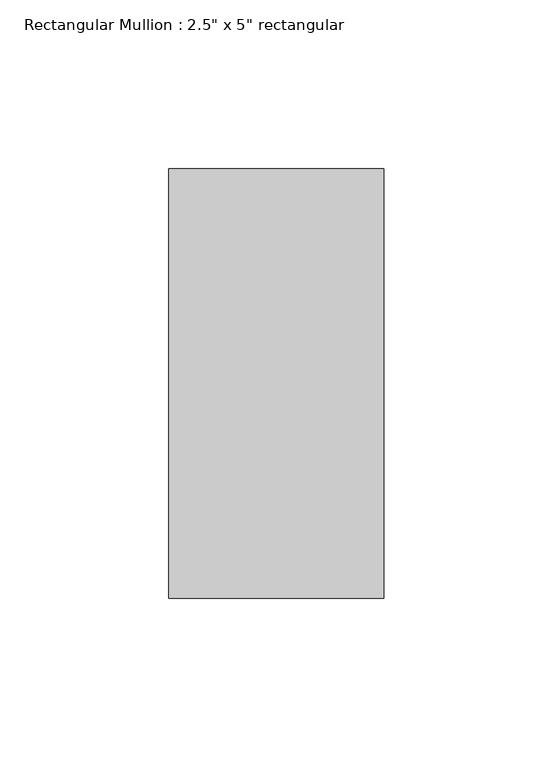
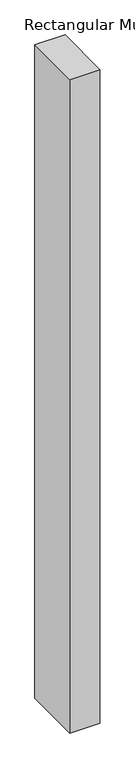
"""IFC4 building model written with IfcOpenShell, lengths in millimetres: member geometry."""

from ifc_helpers import new_model, si_unit, frame, origin, place, context, project, spatial, polyline, outline, extrude, source, transform, mapped, element, save


def member_b9522cbe(model_context):
    return source(origin(), model_context, "Body", "SweptSolid", [
        extrude(outline(polyline([(0.0, 63.5), (0.0, -63.5), (-63.5, -63.5), (-63.5, 63.5), (0.0, 63.5)])), frame((0.0, 0.0, -1452.5193485), z_axis=(0.0, 0.0, 1.0), x_axis=(1.0, 0.0, 0.0)), (0.0, 0.0, 1.0), 1452.5193485),
    ])


if __name__ == "__main__":
    model = new_model("IFC4")
    model_context = context("Model", 3, world=origin())
    ifc_project = project(units=[si_unit("LENGTHUNIT", "METRE", prefix="MILLI")], contexts=[model_context])
    site = spatial("IfcSite", under=ifc_project)
    building = spatial("IfcBuilding", under=site)
    placement = place(None, origin())
    member_shape = member_b9522cbe(model_context)
    element("IfcMember", 1, ObjectType="Rectangular Mullion : 2.5\" x 5\" rectangular", at=placement, inside=building, context=model_context, shape_type="MappedRepresentation", body=[
        mapped(member_shape, transform((0.0, 0.0, 0.0), x_axis=(1.0, 0.0, 0.0), y_axis=(0.0, 1.0, 0.0), z_axis=(0.0, 0.0, 1.0))),
    ])
    save(model, "model.ifc")

# Revit data of these elements
# Type "Rectangular Mullion : 2.5\" x 5\" rectangular"
#   built-in parameter 1007304 = 0.416667 (stored number, unit not read)
#   built-in parameter 1007301 = 0.104167 (stored number, unit not read)
#   built-in parameter 1007300 = 0.104167 (stored number, unit not read)
# Element 1 (IfcMember, "Rectangular Mullion : 2.5\" x 5\" rectangular")
#   Materials on its faces: "Aluminum"
# Materials
#   "Aluminum": class "Metal", colour RGB 247 247 247, transparency 0, Description = "Aluminum 6061", Cost = 0
